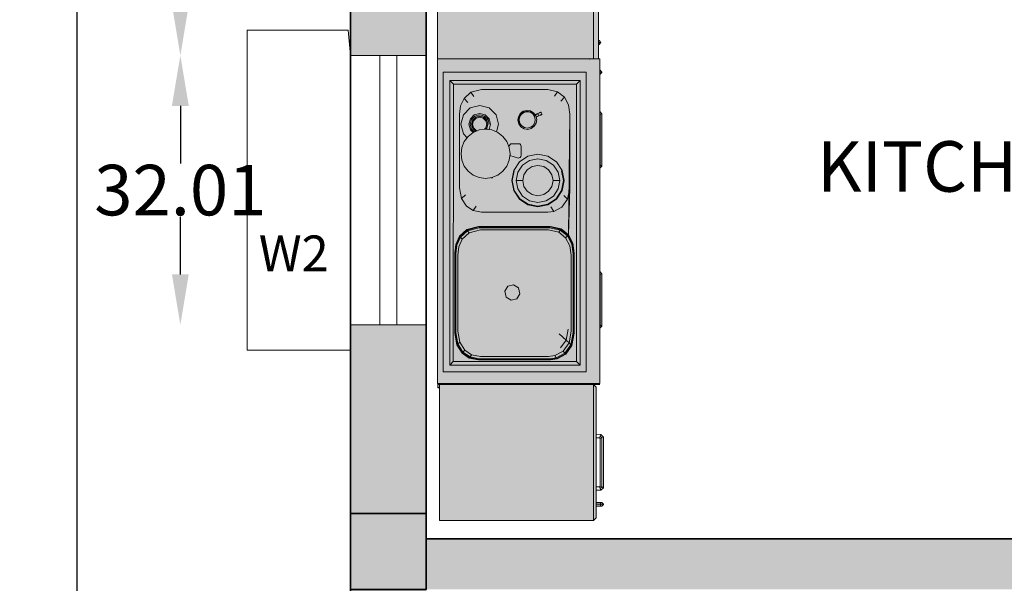
# Model space of a CAD drawing. Units: inches. Extents: x 1994 to 3075, y 3517 to 3950.
# Tile 49 of 58: x 2630 to 2747, y 3656 to 3723. Entities that reach past the tile are written whole.
import ezdxf

# ---------------------------------------------------------------- set-up
doc = ezdxf.new("R2010")
doc.units = ezdxf.units.IN
for name, color, linetype, lineweight in [('A-ANNO-DIMS', 2, 'Continuous', 18), ('A-ANNO-TEXT', 7, 'Continuous', 18), ('A-COLS', 7, 'Continuous', 35), ('A-COLS-PATT', 6, 'Continuous', 13), ('A-FLOR-FIXT', 8, 'Continuous', 18), ('A-GLAZ', 4, 'Continuous', 18), ('A-GLAZ-PROJ', 4, 'Continuous', 18), ('A-WALL', 7, 'Continuous', 35), ('A-WALL-PATT', 252, 'Continuous', 13)]:
    doc.layers.add(name, color=color, linetype=linetype, lineweight=lineweight)
doc.layers.add('hatch', color=254, linetype='Continuous')
doc.styles.get("Standard").update_dxf_attribs({"font": 'arial.ttf'})
doc.dimstyles.get("Standard").update_dxf_attribs({"dimtxt": 6, "dimasz": 6, "dimexe": 0.18, "dimexo": 0.0625, "dimgap": 0.09, "dimtad": 0, "dimtih": 1, "dimtoh": 1, "dimdec": 4, "dimzin": 0, "dimdsep": 46, "dimlunit": 4, "dimtxsty": 'Standard', "dimcen": 0.09, "dimse1": 1, "dimse2": 1, "dimadec": 0, "dimazin": 0, "dimtfac": 1, "dimtdec": 4, "dimtofl": 0, "dimtmove": 0, "dimatfit": 3, "dimfxl": 1, "dimtolj": 1, "dimtzin": 0, "dimarcsym": 0})

# ---------------------------------------------------------------- blocks, each defined once
blk = doc.blocks.new('kithen1')
at = {"layer": 'hatch'}
blk.add_hatch(color=256, dxfattribs=at).paths.add_polyline_path([(-2799.7, -8.3), (-2273.3, -8.3), (-2273.3, -1.7), (-2257.5, -1.7), (-2257.5, -1.1), (-1023.7, -1.1), (-1023.7, 0), (0, 0), (0, -0.3), (0.3, -0.3), (0.3, -1009.9), (-6.1, -1009.9), (-6.1, -2189.3), (-615.8, -2189.3), (-626.5, -2178.9), (-626.5, -1578.2), (-615.8, -1567.8), (-649.5, -1567.8), (-649.5, -1399.1), (-650.3, -1399.1), (-650.3, -1376.8), (-657.9, -1368.5), (-657.8, -1162.4), (-650.3, -1155.1), (-650.3, -1126.4), (-649.5, -1126.4), (-649.5, -1081.1), (-650.3, -1081.1), (-650.3, -1021.1), (-649.5, -1021.1), (-649.5, -959.1), (-651, -959.1), (-650.7, -903), (-653.5, -903), (-660.6, -895.5), (-660.5, -894.6), (-653.5, -887.1), (-651, -887.1), (-651, -638.7), (-651.2, -638.5), (-898.3, -638.5), (-898.3, -640.4), (-905.9, -647.4), (-906.8, -647.4), (-914.3, -640.4), (-914.3, -638.5), (-971.4, -638.5), (-971.4, -642.6), (-1016.2, -642.6), (-1016.2, -643.9), (-1023.8, -650.9), (-1024.7, -650.9), (-1032.2, -643.9), (-1032.2, -642.6), (-1179.7, -642.6), (-1188.8, -650.9), (-1395.6, -650.9), (-1403.7, -642.6), (-1813.5, -642.6), (-1822.6, -650.9), (-2029.4, -650.9), (-2037.5, -642.6), (-2257.5, -642.6), (-2257.5, -618.1), (-2261.3, -618.1), (-2271.7, -628.7), (-2458, -628.7), (-2727.7, -628.7), (-2727.7, -651.1), (-2735, -658.1), (-2735.9, -658), (-2743.2, -651.1), (-2743.2, -628.7), (-2789.4, -628.7), (-2799.7, -618.1)])
at = {"color": 0}
for p, q in [((0, 0), (-1023.7, 0)), ((-2261.3, -8.3), (-2799.7, -8.3)), ((-2799.7, -8.3), (-2799.7, -618.1)), ((-2273.3, -1.9), (-2273.9, -1.9)), ((-2273.9, -1.9), (-2273.9, -8.3)), ((-2261.3, -1.7), (-2273.3, -1.7)), ((-2273.3, -1.7), (-2273.3, -8.3)), ((-2261.3, -601.6), (-2261.3, -1.7)), ((-2261.3, -618.1), (-2261.3, -8.3)), ((-2261, -8.5), (-2261.3, -8.5)), ((-971.4, -1.1), (-2257.5, -1.1)), ((-2257.5, -1.1), (-2257.5, -642.6)), ((-1023.7, -22.5), (-2210.1, -22.5)), ((-2210.1, -22.5), (-2210.1, -589.1)), ((-1023.7, -589.1), (-1023.7, -22.5)), ((-971.4, -1.1), (-971.4, -600.9)), ((-2257.5, -51.5), (-2261.3, -51.5)), ((-2261.3, -51.5), (-2261.3, -536.3)), ((-2183.7, -48.8), (-1056.9, -48.9)), ((-2169.4, -62.7), (-2183.7, -48.8)), ((-2183.7, -48.8), (-2183.7, -565)), ((-2169.7, -550.2), (-2169.4, -62.7)), ((-1071, -63.6), (-2169.4, -62.7)), ((-2103.6, -76.6), (-2136.6, -97.6)), ((-2057.7, -68.5), (-2103.6, -76.6)), ((-2102.3, -78.1), (-2056.8, -70)), ((-2055, -72.6), (-2100.1, -80.6)), ((-1740.9, -68.5), (-2057.7, -68.5)), ((-2056.8, -70), (-1741.9, -70)), ((-1743.7, -72.6), (-2055, -72.6)), ((-1709.7, -76.9), (-1743.7, -72.6)), ((-1741.9, -70), (-1707.6, -74.4)), ((-1706.4, -72.9), (-1740.9, -68.5)), ((-1678, -91.5), (-1709.7, -76.9)), ((-1707.6, -74.4), (-1675.5, -89.1)), ((-1674.1, -87.7), (-1706.4, -72.9)), ((-1056.9, -48.9), (-1071, -63.6)), ((-1071, -550.2), (-1071, -63.6)), ((-1056.9, -48.9), (-1056.9, -565)), ((-2136.6, -97.6), (-2156.1, -126.2)), ((-2154.5, -127.3), (-2135.1, -98.9)), ((-2132.5, -101.2), (-2151.7, -129.3)), ((-2124.5, -108.2), (-2143, -135.3)), ((-2135.1, -98.9), (-2102.3, -78.1)), ((-2132.5, -101.2), (-2135.1, -98.9)), ((-2100.1, -80.6), (-2132.5, -101.2)), ((-2124.5, -108.2), (-2132.5, -101.2)), ((-2093.2, -88.3), (-2124.5, -108.2)), ((-2100.1, -80.6), (-2102.3, -78.1)), ((-2093.2, -88.3), (-2100.1, -80.6)), ((-2049.7, -80.6), (-2093.2, -88.3)), ((-1749, -80.6), (-2049.7, -80.6)), ((-1716.2, -84.8), (-1749, -80.6)), ((-1685.6, -98.8), (-1716.2, -84.8)), ((-1678, -91.5), (-1685.6, -98.8)), ((-1685.6, -98.8), (-1660.4, -125.8)), ((-1651.9, -119.5), (-1678, -91.5)), ((-1675.5, -89.1), (-1649.1, -117.4)), ((-1647.6, -116.2), (-1674.1, -87.7)), ((-1635.3, -163.2), (-1647.6, -116.2)), ((-1554, -114.9), (-1572, -141.2)), ((-1523.7, -95.6), (-1554, -114.9)), ((-1481.5, -88.1), (-1523.7, -95.6)), ((-1523.7, -95.6), (-1509.8, -111.1)), ((-1189.8, -88.1), (-1481.5, -88.1)), ((-1416.2, -122.1), (-1396, -106.6)), ((-1396, -106.6), (-1372.5, -96.9)), ((-1372.5, -96.9), (-1347.3, -93.6)), ((-1347.3, -93.6), (-1322, -96.9)), ((-1322, -96.9), (-1298.5, -106.6)), ((-1298.5, -106.6), (-1278.3, -122.1)), ((-1283.4, -118.2), (-1268.1, -102.9)), ((-1268.1, -102.9), (-1230.5, -92.9)), ((-1230.5, -92.9), (-1193, -102.9)), ((-1193, -102.9), (-1165.5, -130.3)), ((-1157.9, -92.2), (-1189.8, -88.1)), ((-1128.2, -105.8), (-1157.9, -92.2)), ((-1143.5, -120.5), (-1128.2, -105.8)), ((-1128.2, -105.8), (-1103.8, -132)), ((-2156.1, -126.2), (-2163.3, -163.2)), ((-2161.7, -164.1), (-2154.5, -127.3)), ((-2151.7, -129.3), (-2158.8, -165.7)), ((-2151.7, -129.3), (-2154.5, -127.3)), ((-2143, -135.3), (-2151.7, -129.3)), ((-2149.9, -170.5), (-2143, -135.3)), ((-1660.4, -125.8), (-1651.9, -119.5)), ((-1648.8, -170.4), (-1660.4, -125.8)), ((-1649.1, -117.4), (-1651.9, -119.5)), ((-1651.9, -119.5), (-1639.9, -165.7)), ((-1649.1, -117.4), (-1637, -164.1)), ((-1572, -141.2), (-1578.6, -175.3)), ((-1572, -141.2), (-1554.6, -153.3)), ((-1441.5, -165.7), (-1431.7, -142.2)), ((-1431.7, -142.2), (-1416.2, -122.1)), ((-1278.3, -122.1), (-1262.8, -142.2)), ((-1252, -130.7), (-1263.1, -141.8)), ((-1262.8, -142.2), (-1253, -165.7)), ((-1249.5, -134.9), (-1261, -146.4)), ((-1258.4, -151.7), (-1258.6, -152.3)), ((-1246.6, -139.9), (-1258.4, -151.7)), ((-1255.2, -153.5), (-1258.4, -151.7)), ((-1255.2, -153.5), (-1256.4, -157.6)), ((-1244.8, -143), (-1255.2, -153.5)), ((-1252, -130.7), (-1230.5, -124.9)), ((-1249.5, -134.9), (-1230.5, -129.8)), ((-1230.5, -135.6), (-1246.6, -139.9)), ((-1246.6, -139.9), (-1244.8, -143)), ((-1244.8, -143), (-1230.5, -139.2)), ((-1230.5, -124.9), (-1209.1, -130.7)), ((-1230.5, -129.8), (-1211.6, -134.9)), ((-1214.5, -139.9), (-1230.5, -135.6)), ((-1230.5, -135.6), (-1230.5, -139.2)), ((-1230.5, -139.2), (-1216.3, -143)), ((-1216.3, -143), (-1214.5, -139.9)), ((-1205.8, -153.5), (-1216.3, -143)), ((-1211.6, -134.9), (-1214.5, -139.9)), ((-1214.5, -139.9), (-1202.7, -151.7)), ((-1211.6, -134.9), (-1197.7, -148.8)), ((-1209.1, -130.7), (-1193.4, -146.3)), ((-1202.7, -151.7), (-1205.8, -153.5)), ((-1205.8, -153.5), (-1202, -167.7)), ((-1198.4, -167.7), (-1202.7, -151.7)), ((-1197.7, -148.8), (-1192.6, -167.7)), ((-1193.4, -146.3), (-1187.6, -167.7)), ((-1165.5, -130.3), (-1155.5, -167.7)), ((-1103.8, -132), (-1120.8, -144.8)), ((-1103.8, -132), (-1092.5, -175.3)), ((-2163.3, -163.2), (-2163.3, -447.5)), ((-2161.7, -446.6), (-2161.7, -164.1)), ((-2158.8, -165.7), (-2158.8, -445)), ((-2149.9, -440.2), (-2149.9, -170.5)), ((-1648.8, -440.2), (-1648.8, -170.4)), ((-1639.9, -165.7), (-1639.9, -445)), ((-1637, -164.1), (-1637, -446.6)), ((-1635.3, -447.4), (-1635.3, -163.2)), ((-1578.6, -175.3), (-1578.6, -437)), ((-1444.8, -190.8), (-1441.5, -165.7)), ((-1441.5, -216), (-1444.8, -190.8)), ((-1253, -165.7), (-1249.7, -190.8)), ((-1249.7, -190.8), (-1253, -216)), ((-1250.2, -186.9), (-1244.8, -192.3)), ((-1246.6, -195.5), (-1249.9, -192.2)), ((-1244.8, -192.3), (-1246.6, -195.5)), ((-1230.5, -196.1), (-1244.8, -192.3)), ((-1216.3, -192.3), (-1230.5, -196.1)), ((-1205.8, -181.9), (-1216.3, -192.3)), ((-1216.3, -192.3), (-1214.5, -195.5)), ((-1214.5, -195.5), (-1202.7, -183.7)), ((-1197.7, -186.6), (-1211.6, -200.5)), ((-1193.4, -189.1), (-1209.1, -204.7)), ((-1202, -167.7), (-1205.8, -181.9)), ((-1205.8, -181.9), (-1202.7, -183.7)), ((-1202.7, -183.7), (-1198.4, -167.7)), ((-1202, -167.7), (-1198.4, -167.7)), ((-1192.6, -167.7), (-1197.7, -186.6)), ((-1187.6, -167.7), (-1193.4, -189.1)), ((-1155.5, -167.7), (-1165.5, -205.1)), ((-1092.5, -175.3), (-1092.5, -437)), ((-1442, -212), (-1442.1, -213.6)), ((-1442.1, -213.6), (-1441.9, -216.3)), ((-1441.9, -216.3), (-1441.5, -218.2)), ((-1431.7, -239.4), (-1441.5, -216)), ((-1441.5, -218.2), (-1440.8, -218.9)), ((-1440.8, -218.9), (-1440.3, -218.9)), ((-1253, -216), (-1262.8, -239.4)), ((-1230.5, -210.4), (-1251.6, -204.8)), ((-1250.8, -199.1), (-1249.5, -200.5)), ((-1230.5, -199.7), (-1246.6, -195.5)), ((-1214.5, -195.5), (-1230.5, -199.7)), ((-1230.5, -196.1), (-1230.5, -199.7)), ((-1211.6, -200.5), (-1230.5, -205.5)), ((-1209.1, -204.7), (-1230.5, -210.4)), ((-1193, -232.5), (-1230.5, -242.5)), ((-1211.6, -200.5), (-1214.5, -195.5)), ((-1165.5, -205.1), (-1193, -232.5)), ((-1914.6, -272.1), (-1926.9, -292)), ((-1891.8, -266.6), (-1914.6, -272.1)), ((-1871.8, -278.8), (-1891.8, -266.6)), ((-1416.2, -259.6), (-1431.7, -239.4)), ((-1396, -275), (-1416.2, -259.6)), ((-1278.3, -259.6), (-1298.5, -275)), ((-1262.8, -239.4), (-1278.3, -259.6)), ((-1230.5, -242.5), (-1260.7, -234.4)), ((-1926.9, -292), (-1921.4, -314.8)), ((-1878.5, -321.5), (-1866.3, -301.6)), ((-1866.3, -301.6), (-1871.8, -278.8)), ((-1526.8, -324.6), (-1493.1, -302.1)), ((-1493.1, -302.2), (-1526.8, -324.6)), ((-1492.2, -304.2), (-1525.2, -326.2)), ((-1493.1, -302.1), (-1453.2, -294.2)), ((-1453.2, -294.3), (-1493.1, -302.2)), ((-1453.2, -296.5), (-1492.2, -304.2)), ((-1453.2, -311.7), (-1486.4, -318.2)), ((-1453.2, -294.2), (-1413.4, -302.1)), ((-1413.4, -302.2), (-1453.2, -294.3)), ((-1453.2, -294.3), (-1453.2, -296.5)), ((-1453.2, -296.5), (-1414.2, -304.2)), ((-1453.2, -311.7), (-1420.1, -318.2)), ((-1453.2, -338.2), (-1453.2, -311.7)), ((-1413.4, -302.1), (-1379.6, -324.6)), ((-1379.6, -324.6), (-1413.4, -302.2)), ((-1372.5, -284.8), (-1396, -275)), ((-1347.3, -288.1), (-1372.5, -284.8)), ((-1364, -321.4), (-1354.5, -287.1)), ((-1322, -284.8), (-1347.3, -288.1)), ((-1298.5, -275), (-1322, -284.8)), ((-1316.5, -282.5), (-1307.2, -290.8)), ((-1307.2, -290.8), (-1307.2, -321.4)), ((-1921.4, -314.8), (-1901.4, -327)), ((-1901.4, -327), (-1878.5, -321.5)), ((-1526.8, -324.6), (-1549.4, -358.3)), ((-1549.4, -358.3), (-1526.8, -324.6)), ((-1525.2, -326.2), (-1547.3, -359.2)), ((-1514.5, -337), (-1533.3, -365)), ((-1486.4, -318.2), (-1514.5, -337)), ((-1495.7, -355.7), (-1476.2, -342.8)), ((-1476.2, -342.8), (-1453.2, -338.2)), ((-1430.3, -342.8), (-1453.2, -338.2)), ((-1410.8, -355.7), (-1430.3, -342.8)), ((-1420.1, -318.2), (-1392, -337)), ((-1392, -337), (-1373.2, -365)), ((-1379.6, -324.6), (-1357, -358.3)), ((-1357, -358.3), (-1379.6, -324.6)), ((-1363.6, -324.3), (-1364, -321.4)), ((-1361.6, -328), (-1363.6, -324.3)), ((-1357.9, -330.6), (-1361.6, -328)), ((-1352.7, -331.6), (-1357.9, -330.6)), ((-1318.5, -331.6), (-1352.7, -331.6)), ((-1314.3, -331), (-1318.5, -331.6)), ((-1310.7, -329.1), (-1314.3, -331)), ((-1308.2, -326), (-1310.7, -329.1)), ((-1307.2, -321.4), (-1308.2, -326)), ((-1250.4, -357.6), (-1248.3, -343.1)), ((-1248.3, -343.1), (-1240.7, -330.6)), ((-1245.1, -357.3), (-1243.2, -344.9)), ((-1243.2, -344.9), (-1236.8, -334.2)), ((-1240.7, -330.6), (-1228.9, -321.9)), ((-1227.6, -324.8), (-1238.3, -332.8)), ((-1236.8, -334.2), (-1226.7, -326.8)), ((-1228.9, -321.9), (-1214.7, -318.4)), ((-1227.6, -324.8), (-1228.3, -323.3)), ((-1214.6, -321.6), (-1227.6, -324.8)), ((-1226.7, -326.8), (-1214.5, -323.7)), ((-1214.7, -318.4), (-1200.3, -320.6)), ((-1214.7, -319.9), (-1214.6, -321.6)), ((-1214.6, -321.6), (-1201.4, -323.6)), ((-1214.5, -323.7), (-1202.1, -325.6)), ((-1202.1, -325.6), (-1191.3, -332)), ((-1201.4, -323.6), (-1200.8, -322)), ((-1201.4, -323.6), (-1189.9, -330.5)), ((-1200.3, -320.6), (-1187.7, -328.1)), ((-1191.3, -332), (-1183.9, -342.1)), ((-1189.9, -330.5), (-1188.7, -329.2)), ((-1189.9, -330.5), (-1181.9, -341.2)), ((-1187.7, -328.1), (-1179, -339.8)), ((-1183.9, -342.1), (-1180.8, -354.2)), ((-1181.9, -341.2), (-1180.4, -340.5)), ((-1181.9, -341.2), (-1178.7, -354.1)), ((-1179, -339.8), (-1175.5, -354)), ((-1549.4, -358.3), (-1557.3, -398)), ((-1557.3, -398), (-1549.4, -358.3)), ((-1547.3, -359.2), (-1555.1, -398)), ((-1533.3, -365), (-1539.9, -398)), ((-1513.2, -398), (-1508.7, -375.1)), ((-1508.7, -375.1), (-1495.7, -355.7)), ((-1397.8, -375.1), (-1410.8, -355.7)), ((-1393.2, -398), (-1397.8, -375.1)), ((-1373.2, -365), (-1366.6, -398)), ((-1357, -358.3), (-1349.1, -398)), ((-1349.1, -398), (-1357, -358.3)), ((-1246.9, -371.7), (-1250.4, -357.6)), ((-1238.2, -383.5), (-1246.9, -371.7)), ((-1242, -369.4), (-1245.1, -357.3)), ((-1234.6, -379.5), (-1242, -369.4)), ((-1225.6, -391), (-1238.2, -383.5)), ((-1223.8, -385.9), (-1234.6, -379.5)), ((-1211.4, -387.8), (-1223.8, -385.9)), ((-1199.2, -384.8), (-1211.4, -387.8)), ((-1197, -389.6), (-1211.2, -393.1)), ((-1189.2, -377.3), (-1199.2, -384.8)), ((-1187.6, -378.8), (-1198.3, -386.7)), ((-1185.2, -380.9), (-1197, -389.6)), ((-1193.3, -386.9), (-1194.2, -387.6)), ((-1193.1, -386.7), (-1193.3, -386.9)), ((-1193.3, -386.9), (-1191.3, -391.2)), ((-1192.7, -386.5), (-1192.9, -386.6)), ((-1192.6, -386.8), (-1192.7, -386.5)), ((-1190.5, -391.2), (-1192.6, -386.8)), ((-1182.7, -366.6), (-1189.2, -377.3)), ((-1180.7, -367.3), (-1187.6, -378.8)), ((-1187.6, -378.8), (-1186.3, -379.9)), ((-1177.6, -368.4), (-1185.2, -380.9)), ((-1180.8, -354.2), (-1182.7, -366.6)), ((-1178.7, -354.1), (-1180.7, -367.3)), ((-1180.7, -367.3), (-1179.1, -367.9)), ((-1178.7, -354.1), (-1177, -354.1)), ((-1175.5, -354), (-1177.6, -368.4)), ((-1557.3, -398), (-1549.4, -437.8)), ((-1549.4, -437.8), (-1557.3, -398)), ((-1555.1, -398), (-1547.3, -436.9)), ((-1539.9, -398), (-1533.3, -431.1)), ((-1508.7, -420.9), (-1513.2, -398)), ((-1495.7, -440.4), (-1508.7, -420.9)), ((-1410.8, -440.4), (-1397.8, -420.9)), ((-1397.8, -420.9), (-1393.2, -398)), ((-1366.6, -398), (-1373.2, -431.1)), ((-1349.1, -398), (-1357, -437.8)), ((-1357, -437.8), (-1349.1, -398)), ((-1211.2, -393.1), (-1225.6, -391)), ((-1202.1, -390.9), (-1202.4, -391)), ((-1202.4, -391), (-1202, -390.9)), ((-1202.4, -391), (-1202.4, -391)), ((-1202.4, -391), (-1202.3, -391.3)), ((-1202.3, -391.3), (-1200.2, -395.7)), ((-1202, -390.9), (-1202.1, -390.9)), ((-1201.7, -390.8), (-1199.7, -395.1)), ((-1200.2, -395.7), (-1199.7, -395.1)), ((-1200.2, -395.7), (-1197.3, -401.8)), ((-1199.7, -395.1), (-1198, -394.1)), ((-1199.7, -395.1), (-1196.7, -401.5)), ((-1197.3, -401.8), (-1196.7, -401.5)), ((-1197.3, -401.8), (-1194.5, -407.8)), ((-1196.7, -401.5), (-1190.1, -398.4)), ((-1196.7, -401.5), (-1193.7, -407.8)), ((-1194.5, -407.8), (-1193.7, -407.8)), ((-1192.4, -412.2), (-1194.5, -407.8)), ((-1193.7, -407.8), (-1191.8, -407.2)), ((-1193.7, -407.8), (-1191.5, -412.5)), ((-1191.3, -391.2), (-1193.2, -391.8)), ((-1191.6, -413.9), (-1192.4, -412.2)), ((-1190.7, -414.2), (-1191.6, -413.9)), ((-1191.3, -391.2), (-1190.5, -391.2)), ((-1188.3, -397.5), (-1191.3, -391.2)), ((-1188.7, -413.8), (-1190.7, -414.2)), ((-1190.5, -391.2), (-1187.6, -397.2)), ((-1190.1, -398.4), (-1188.3, -397.5)), ((-1186.2, -412.8), (-1188.7, -413.8)), ((-1187.6, -397.2), (-1188.3, -397.5)), ((-1188.3, -397.5), (-1185.3, -403.9)), ((-1184.8, -403.3), (-1187.6, -397.2)), ((-1185.3, -403.9), (-1186.9, -404.9)), ((-1183.8, -411.5), (-1186.2, -412.8)), ((-1185.3, -403.9), (-1184.8, -403.3)), ((-1183.1, -408.5), (-1185.3, -403.9)), ((-1184.8, -403.3), (-1182.7, -407.7)), ((-1182.3, -410.2), (-1183.8, -411.5)), ((-1182.7, -407.7), (-1181.9, -409.3)), ((-1181.9, -409.3), (-1182.3, -410.2)), ((-2163.3, -447.5), (-2159.9, -473.6)), ((-2158.2, -472.6), (-2161.7, -446.6)), ((-2158.8, -445), (-2155.4, -470.7)), ((-2155.4, -470.7), (-2146.6, -465)), ((-2146.6, -465), (-2149.9, -440.2)), ((-2146.6, -465), (-2128.8, -498)), ((-1658, -480.4), (-1648.8, -440.2)), ((-1639.9, -445), (-1649.4, -486.6)), ((-1637, -446.6), (-1646.6, -488.6)), ((-1645, -489.8), (-1635.3, -447.4)), ((-1578.6, -437), (-1575.5, -461.1)), ((-1575.5, -461.1), (-1557.8, -449.7)), ((-1575.5, -461.1), (-1558.2, -493)), ((-1549.4, -437.8), (-1526.8, -471.4)), ((-1526.8, -471.4), (-1549.4, -437.8)), ((-1547.3, -436.9), (-1525.2, -469.8)), ((-1533.3, -431.1), (-1514.5, -459.1)), ((-1514.5, -459.1), (-1486.4, -477.9)), ((-1476.2, -453.3), (-1495.7, -440.4)), ((-1453.2, -457.9), (-1476.2, -453.3)), ((-1453.2, -457.9), (-1430.3, -453.3)), ((-1453.2, -484.4), (-1453.2, -457.9)), ((-1430.3, -453.3), (-1410.8, -440.4)), ((-1392, -459.1), (-1420.1, -477.9)), ((-1373.2, -431.1), (-1392, -459.1)), ((-1357, -437.8), (-1379.6, -471.4)), ((-1379.6, -471.4), (-1357, -437.8)), ((-1101.4, -476), (-1118.7, -463.5)), ((-1092.5, -437), (-1101.4, -476)), ((-2159.9, -473.6), (-2141.1, -508.3)), ((-2139.6, -507.1), (-2158.2, -472.6)), ((-2137, -504.8), (-2155.4, -470.7)), ((-2137, -504.8), (-2139.6, -507.1)), ((-2128.8, -498), (-2137, -504.8)), ((-2103.3, -528.8), (-2137, -504.8)), ((-2128.8, -498), (-2096.3, -521.1)), ((-2085.5, -509.3), (-2116.3, -487.4)), ((-2060.9, -482.3), (-2085.5, -509.3)), ((-1680.2, -507.9), (-1658, -480.4)), ((-1649.4, -486.6), (-1672.5, -515.1)), ((-1646.6, -488.6), (-1669.9, -517.4)), ((-1668.5, -518.8), (-1645, -489.8)), ((-1649.4, -486.6), (-1658, -480.4)), ((-1646.6, -488.6), (-1649.4, -486.6)), ((-1558.2, -493), (-1526.7, -515.5)), ((-1493.1, -493.9), (-1526.8, -471.4)), ((-1526.8, -471.4), (-1493.1, -493.9)), ((-1526.7, -515.5), (-1512.6, -500.1)), ((-1525.2, -469.8), (-1492.2, -491.9)), ((-1453.2, -501.8), (-1493.1, -493.9)), ((-1493.1, -493.9), (-1453.2, -501.8)), ((-1492.2, -491.9), (-1453.2, -499.6)), ((-1486.4, -477.9), (-1453.2, -484.4)), ((-1420.1, -477.9), (-1453.2, -484.4)), ((-1453.2, -499.6), (-1414.2, -491.9)), ((-1413.4, -493.9), (-1453.2, -501.8)), ((-1453.2, -501.8), (-1413.4, -493.9)), ((-1453.2, -499.6), (-1453.2, -501.8)), ((-1379.6, -471.4), (-1413.4, -493.9)), ((-1413.4, -493.9), (-1379.6, -471.4)), ((-1123, -502.7), (-1153.4, -518.8)), ((-1123, -502.7), (-1138.7, -488.2)), ((-1101.4, -476), (-1123, -502.7)), ((-2257.5, -535.3), (-2257.9, -535.3)), ((-2141.1, -508.3), (-2106.9, -532.7)), ((-2105.6, -531.3), (-2139.6, -507.1)), ((-2106.9, -532.7), (-2057.7, -542.2)), ((-2103.3, -528.8), (-2105.6, -531.3)), ((-2056.8, -540.7), (-2105.6, -531.3)), ((-2096.3, -521.1), (-2103.3, -528.8)), ((-2055, -538.1), (-2103.3, -528.8)), ((-2096.3, -521.1), (-2085.5, -509.3)), ((-2049.7, -530.1), (-2096.3, -521.1)), ((-2085.5, -509.3), (-2041.5, -517.8)), ((-2057.7, -542.2), (-2056.8, -540.7)), ((-1783.5, -542.2), (-2057.7, -542.2)), ((-1781.7, -540.7), (-2056.8, -540.7)), ((-1778.6, -538.1), (-2055, -538.1)), ((-1749, -530.1), (-2049.7, -530.1)), ((-1749, -530.1), (-1797.1, -530.1)), ((-1743.7, -538.1), (-1797.1, -538.1)), ((-1741.9, -540.7), (-1797.1, -540.7)), ((-1740.9, -542.2), (-1797.1, -542.2)), ((-1711.5, -524.5), (-1749, -530.1)), ((-1704.9, -532.3), (-1743.7, -538.1)), ((-1741.9, -540.7), (-1702.7, -534.9)), ((-1740.9, -542.2), (-1741.9, -540.7)), ((-1701.5, -536.3), (-1740.9, -542.2)), ((-1680.2, -507.9), (-1711.5, -524.5)), ((-1672.5, -515.1), (-1704.9, -532.3)), ((-1702.7, -534.9), (-1669.9, -517.4)), ((-1668.5, -518.8), (-1701.5, -536.3)), ((-1672.5, -515.1), (-1680.2, -507.9)), ((-1669.9, -517.4), (-1672.5, -515.1)), ((-1189.8, -524.2), (-1668.5, -518.8)), ((-1481.5, -524.2), (-1668.5, -518.8)), ((-1526.7, -515.5), (-1481.5, -524.2)), ((-1189.8, -524.2), (-1481.5, -524.2)), ((-1153.4, -518.8), (-1189.8, -524.2)), ((-2183.7, -565), (-2169.7, -550.2)), ((-1797.1, -565), (-2183.7, -565)), ((-1793.1, -550.2), (-2169.7, -550.2)), ((-1071, -550.2), (-1797.1, -550.2)), ((-1056.9, -565), (-1797.1, -565)), ((-1056.9, -565), (-1071, -550.2)), ((-2799.7, -618.1), (-2261.3, -618.1)), ((-2789.4, -628.7), (-2799.7, -618.1)), ((-2261.3, -618.1), (-2271.7, -628.7)), ((-2261, -596.4), (-2261.3, -596.4)), ((-2261.3, -626.3), (-2261.3, -601.6)), ((-2210.1, -589.1), (-1789.4, -589.1)), ((-1797.1, -589.1), (-1023.7, -589.1)), ((-972.7, -601.6), (-972.7, -603)), ((-971.4, -600.6), (-971.4, -601.6)), ((-971.4, -603), (-971.4, -642.6)), ((-630.9, -618.1), (-971.4, -618.1)), ((-2271.7, -628.7), (-2789.4, -628.7)), ((-2743.2, -628.7), (-2743.2, -644.8)), ((-2743.2, -644.8), (-2742.3, -644.5)), ((-2743.2, -651.1), (-2743.2, -644.8)), ((-2742.3, -650.3), (-2743.2, -651.1)), ((-2742.3, -651.1), (-2743.2, -651.1)), ((-2743.2, -651.1), (-2735.9, -658)), ((-2742.3, -628.7), (-2742.3, -644.4)), ((-2742.3, -644.4), (-2734.9, -647.4)), ((-2742.3, -644.4), (-2742.3, -651.1)), ((-2735, -658.1), (-2742.3, -651.1)), ((-2735.9, -658), (-2735, -658.1)), ((-2734.9, -647.4), (-2735, -658.1)), ((-2735, -658.1), (-2727.7, -651.1)), ((-2734.9, -647.4), (-2734.9, -628.7)), ((-2727.7, -644.4), (-2734.9, -647.4)), ((-2727.7, -628.7), (-2727.7, -644.4)), ((-2727.7, -651.1), (-2727.7, -644.4)), ((-2679.7, -628.7), (-2679.4, -647.7)), ((-2679.4, -647.7), (-2665.9, -642)), ((-2669.5, -658), (-2679.4, -647.7)), ((-2666.7, -651.1), (-2672.6, -644.8)), ((-2666.7, -651.1), (-2669.5, -658)), ((-2669.5, -658), (-2469.7, -658.1)), ((-2663.9, -644.2), (-2666.7, -651.1)), ((-2472.3, -651.1), (-2666.7, -651.1)), ((-2665.6, -628.7), (-2665.9, -642)), ((-2665.9, -642), (-2663.9, -644.2)), ((-2663.9, -644.2), (-2474.9, -644.1)), ((-2474.9, -644.1), (-2471.7, -641.3)), ((-2474.9, -644.1), (-2472.3, -651.1)), ((-2472.3, -651.1), (-2465, -644.4)), ((-2469.7, -658.1), (-2472.3, -651.1)), ((-2471.7, -641.3), (-2472, -628.7)), ((-2458.4, -647.4), (-2471.7, -641.3)), ((-2458.4, -647.4), (-2469.7, -658.1)), ((-2458, -628.7), (-2458.4, -647.4)), ((-2261.3, -643.6), (-2261.3, -626.3)), ((-2257.5, -642.6), (-1797.1, -642.6)), ((-2037.5, -642.6), (-2029.4, -650.9)), ((-2029.4, -650.9), (-2026.5, -643.9)), ((-2029.4, -650.9), (-1828.9, -650.9)), ((-2026.5, -643.9), (-2027.8, -642.6)), ((-2025.9, -642.6), (-2026.5, -643.9)), ((-2026.5, -643.9), (-1828.9, -643.9)), ((-1825.3, -643.9), (-1828.9, -643.9)), ((-1822.6, -650.9), (-1828.9, -650.9)), ((-1825.8, -642.6), (-1825.3, -643.9)), ((-1825.3, -643.9), (-1823.8, -642.6)), ((-1822.6, -650.9), (-1825.3, -643.9)), ((-1813.5, -642.6), (-1822.6, -650.9)), ((-971.4, -642.6), (-1797.1, -642.6)), ((-1395.6, -650.9), (-1403.7, -642.6)), ((-1392.7, -643.9), (-1395.6, -650.9)), ((-1395.6, -650.9), (-1188.8, -650.9)), ((-1394, -642.6), (-1392.7, -643.9)), ((-1392.7, -643.9), (-1392.1, -642.6)), ((-1191.5, -643.9), (-1392.7, -643.9)), ((-1192, -642.6), (-1191.5, -643.9)), ((-1191.5, -643.9), (-1190, -642.6)), ((-1188.8, -650.9), (-1191.5, -643.9)), ((-1179.7, -642.6), (-1188.8, -650.9)), ((-1032.2, -643.9), (-1032.2, -642.6)), ((-1031.4, -643.1), (-1032.2, -643.9)), ((-1031.4, -643.9), (-1032.2, -643.9)), ((-1032.2, -643.9), (-1024.7, -650.9)), ((-1031.4, -642.6), (-1031.4, -643.9)), ((-1023.8, -650.9), (-1031.4, -643.9)), ((-1024.7, -650.9), (-1023.8, -650.9)), ((-1023.8, -650.9), (-1023.8, -642.6)), ((-1016.2, -643.9), (-1023.8, -650.9)), ((-1016.2, -642.6), (-1016.2, -643.9)), ((-971.4, -635.7), (-971.4, -641.8)), ((-971.4, -641.8), (-971.4, -638.3)), ((-651.2, -638.5), (-971.4, -638.5)), ((-914.3, -640.4), (-914.4, -638.5)), ((-913.5, -639.6), (-914.3, -640.4)), ((-913.5, -640.4), (-914.3, -640.4)), ((-914.3, -640.4), (-906.8, -647.3)), ((-913.5, -638.5), (-913.5, -640.4)), ((-905.9, -647.4), (-913.5, -640.4)), ((-906.8, -647.3), (-905.9, -647.4)), ((-905.9, -647.4), (-905.9, -638.5)), ((-898.3, -640.4), (-905.9, -647.4)), ((-898.3, -638.5), (-898.3, -640.4))]:
    blk.add_line(p, q, dxfattribs=at)
for points in [[(-2799.7, -8.3), (-2273.3, -8.3), (-2273.3, -1.7), (-2257.5, -1.7), (-2257.5, -1.1), (-1023.7, -1.1), (-1023.7, 0), (0, 0)], [(-651.2, -638.5), (-898.3, -638.5), (-898.3, -640.4), (-905.9, -647.4), (-906.8, -647.4), (-914.3, -640.4), (-914.3, -638.5), (-971.4, -638.5), (-971.4, -642.6), (-1016.2, -642.6), (-1016.2, -643.9), (-1023.8, -650.9), (-1024.7, -650.9), (-1032.2, -643.9), (-1032.2, -642.6), (-1179.7, -642.6), (-1188.8, -650.9), (-1395.6, -650.9), (-1403.7, -642.6), (-1813.5, -642.6), (-1822.6, -650.9), (-2029.4, -650.9), (-2037.5, -642.6), (-2257.5, -642.6), (-2257.5, -618.1), (-2261.3, -618.1), (-2271.7, -628.7), (-2458, -628.7), (-2727.7, -628.7), (-2727.7, -651.1), (-2735, -658.1), (-2735.9, -658), (-2743.2, -651.1), (-2743.2, -628.7), (-2789.4, -628.7), (-2799.7, -618.1), (-2799.7, -8.3)]]:
    blk.add_lwpolyline(points)
blk = doc.blocks.new('*D29')
at = {"layer": 'A-ANNO-DIMS', "color": 0, "lineweight": -2, "transparency": 16777216}
for p, q in [((2757.66, 3741.43), (2757.66, 3708.56)), ((2757.66, 3669.3), (2757.66, 3702.17))]:
    blk.add_line(p, q, dxfattribs=at)
at = {"layer": 'A-ANNO-DIMS', "color": 0, "transparency": 16777216}
for points in [[(2756.66, 3741.43), (2758.66, 3741.43), (2757.66, 3747.43)], [(2756.66, 3669.3), (2758.66, 3669.3), (2757.66, 3663.3)]]:
    blk.add_solid(points, dxfattribs=at)
at = {"layer": 'Defpoints', "color": 0, "transparency": 16777216}
for p in [(2745.04, 3747.43), (2757.66, 3747.43), (2745.04, 3663.3)]:
    blk.add_point(p, dxfattribs=at)
at = {"layer": 'A-ANNO-DIMS', "color": 0, "transparency": 16777216, "insert": (2757.66, 3705.36), "char_height": 6, "attachment_point": 5}
blk.add_mtext('\\A1;KITCHEN UNIT 84', dxfattribs=at)
blk = doc.blocks.new('*D32')
at = {"layer": 'A-ANNO-DIMS', "color": 0, "lineweight": -2, "transparency": 16777216}
for p, q in [((2636.61, 3908.13), (2636.61, 3730.78)), ((2636.61, 3547.13), (2636.61, 3724.47))]:
    blk.add_line(p, q, dxfattribs=at)
at = {"layer": 'A-ANNO-DIMS', "color": 0, "transparency": 16777216}
for points in [[(2635.61, 3908.13), (2637.61, 3908.13), (2636.61, 3914.13)], [(2635.61, 3547.13), (2637.61, 3547.13), (2636.61, 3541.13)]]:
    blk.add_solid(points, dxfattribs=at)
at = {"layer": 'Defpoints', "color": 0, "transparency": 16777216}
for p in [(2636.61, 3914.13), (2669.07, 3914.13), (2810.07, 3541.13)]:
    blk.add_point(p, dxfattribs=at)
at = {"layer": 'A-ANNO-DIMS', "color": 0, "transparency": 16777216, "insert": (2636.61, 3727.63), "char_height": 6, "attachment_point": 5}
blk.add_mtext('\\A1;373', dxfattribs=at)
blk = doc.blocks.new('*D45')
at = {"layer": 'A-ANNO-DIMS', "color": 0, "lineweight": -2, "transparency": 16777216}
for p, q in [((2648.87, 3712.55), (2648.87, 3705.7)), ((2648.87, 3692.54), (2648.87, 3699.39))]:
    blk.add_line(p, q, dxfattribs=at)
at = {"layer": 'A-ANNO-DIMS', "color": 0, "transparency": 16777216}
for points in [[(2647.87, 3712.55), (2649.87, 3712.55), (2648.87, 3718.55)], [(2647.87, 3692.54), (2649.87, 3692.54), (2648.87, 3686.54)]]:
    blk.add_solid(points, dxfattribs=at)
at = {"layer": 'Defpoints', "color": 0, "transparency": 16777216}
for p in [(2648.87, 3718.55), (2669.07, 3718.55), (2669.07, 3686.54)]:
    blk.add_point(p, dxfattribs=at)
at = {"layer": 'A-ANNO-DIMS', "color": 0, "transparency": 16777216, "insert": (2648.87, 3702.55), "char_height": 6, "attachment_point": 5}
blk.add_mtext('\\A1;32.01', dxfattribs=at)
blk = doc.blocks.new('*D46')
at = {"layer": 'A-ANNO-DIMS', "color": 0, "lineweight": -2, "transparency": 16777216}
for p, q in [((2648.87, 3749.13), (2648.87, 3740)), ((2648.87, 3724.55), (2648.87, 3733.68))]:
    blk.add_line(p, q, dxfattribs=at)
at = {"layer": 'A-ANNO-DIMS', "color": 0, "transparency": 16777216}
for points in [[(2647.87, 3749.13), (2649.87, 3749.13), (2648.87, 3755.13)], [(2647.87, 3724.55), (2649.87, 3724.55), (2648.87, 3718.55)]]:
    blk.add_solid(points, dxfattribs=at)
at = {"layer": 'Defpoints', "color": 0, "transparency": 16777216}
for p in [(2648.87, 3755.13), (2669.07, 3755.13), (2669.07, 3718.55)]:
    blk.add_point(p, dxfattribs=at)
at = {"layer": 'A-ANNO-DIMS', "color": 0, "transparency": 16777216, "insert": (2648.87, 3736.84), "char_height": 6, "attachment_point": 5}
blk.add_mtext('\\A1;36.575', dxfattribs=at)

msp = doc.modelspace()

# ---------------------------------------------------------------- hatches: boundary and pattern name
at = {"layer": 'A-COLS-PATT'}
h = msp.add_hatch(color=256, dxfattribs=at)
h.dxf.hatch_style = 1
h.paths.add_polyline_path([(2678.072, 3914.1269), (2669.072, 3914.1269), (2669.072, 3905.1269), (2678.072, 3905.1269)])
h.paths.add_polyline_path([(2816.072, 3914.1269), (2807.072, 3914.1269), (2807.072, 3905.1269), (2816.072, 3905.1269)])
h.paths.add_polyline_path([(2894.9096, 3914.1269), (2885.9096, 3914.1269), (2885.9096, 3905.1269), (2894.9096, 3905.1269)])
h.paths.add_polyline_path([(3033.072, 3914.1269), (3024.072, 3914.1269), (3024.072, 3905.1269), (3033.072, 3905.1269)])
h.paths.add_polyline_path([(3033.072, 3764.1269), (3024.072, 3764.1269), (3024.072, 3755.1269), (3033.072, 3755.1269)])
h.paths.add_polyline_path([(2895.072, 3764.1269), (2886.072, 3764.1269), (2886.072, 3755.1269), (2895.072, 3755.1269)])
h.paths.add_polyline_path([(2816.072, 3764.1269), (2807.072, 3764.1269), (2807.072, 3755.1269), (2816.072, 3755.1269)])
h.paths.add_polyline_path([(2678.072, 3764.1269), (2669.072, 3764.1269), (2669.072, 3755.1269), (2678.072, 3755.1269)])
h.paths.add_polyline_path([(2678.072, 3664.1269), (2669.072, 3664.1269), (2669.072, 3655.1269), (2678.072, 3655.1269)])
h.paths.add_polyline_path([(2816.072, 3664.1269), (2807.072, 3664.1269), (2807.072, 3655.1269), (2816.072, 3655.1269)])
h.paths.add_polyline_path([(3033.072, 3616.1269), (3024.072, 3616.1269), (3024.072, 3607.1269), (3033.072, 3607.1269)])
h.paths.add_polyline_path([(2894.9096, 3616.1269), (2885.9096, 3616.1269), (2885.9096, 3607.1269), (2894.9096, 3607.1269)])
h.paths.add_polyline_path([(2816.072, 3559.1269), (2807.072, 3559.1269), (2807.072, 3550.1269), (2816.072, 3550.1269)])
h.paths.add_polyline_path([(2678.072, 3559.1269), (2669.072, 3559.1269), (2669.072, 3550.1269), (2678.072, 3550.1269)])
at = {"layer": 'A-WALL-PATT'}
h = msp.add_hatch(color=256, dxfattribs=at)
h.dxf.hatch_style = 1
h.paths.add_polyline_path([(2678.072, 3755.1269), (2669.072, 3755.1269), (2669.072, 3718.5523), (2678.072, 3718.5523)])
h.paths.add_polyline_path([(2807.072, 3761.1269), (2678.072, 3761.1269), (2678.072, 3755.1269), (2807.072, 3755.1269)])
h.paths.add_polyline_path([(2678.072, 3812.7371), (2669.072, 3812.7371), (2669.072, 3809.7371), (2669.072, 3764.1269), (2678.072, 3764.1269)])
h.paths.add_polyline_path([(2678.072, 3905.1269), (2669.072, 3905.1269), (2669.072, 3868.7491), (2678.072, 3868.7491)])
h.paths.add_polyline_path([(2723.826, 3914.1269), (2720.826, 3914.1269), (2678.072, 3914.1269), (2678.072, 3905.1269), (2723.826, 3905.1269)])
h.paths.add_polyline_path([(2807.072, 3914.1269), (2779.838, 3914.1269), (2779.838, 3905.1269), (2807.072, 3905.1269)])
h.paths.add_polyline_path([(2837.6979, 3914.1269), (2834.6979, 3914.1269), (2820.9062, 3914.1269), (2816.072, 3914.1269), (2816.072, 3905.1269), (2837.6979, 3905.1269)])
h.paths.add_polyline_path([(2885.9096, 3914.1269), (2869.71, 3914.1269), (2869.71, 3905.1269), (2876.9183, 3905.1269), (2885.9096, 3905.1269)])
h.paths.add_polyline_path([(2933.6904, 3914.1269), (2930.6904, 3914.1269), (2894.9096, 3914.1269), (2894.9096, 3905.1269), (2933.6904, 3905.1269)])
h.paths.add_polyline_path([(3024.072, 3914.1269), (2989.7025, 3914.1269), (2989.7025, 3905.1269), (3024.072, 3905.1269)])
h.paths.add_polyline_path([(3033.072, 3905.1269), (3024.072, 3905.1269), (3024.072, 3861.4192), (3033.072, 3861.4192)])
h.paths.add_polyline_path([(3033.072, 3805.4072), (3024.072, 3805.4072), (3024.072, 3764.1269), (3033.072, 3764.1269)])
h.paths.add_polyline_path([(3033.072, 3755.1269), (3024.072, 3755.1269), (3024.072, 3732.1247), (3033.072, 3732.1247), (3033.072, 3735.1247)])
h.paths.add_polyline_path([(3024.072, 3761.1269), (2895.072, 3761.1269), (2895.072, 3755.1269), (3024.072, 3755.1269)])
h.paths.add_polyline_path([(3033.072, 3676.1126), (3024.072, 3676.1126), (3024.072, 3616.1269), (3033.072, 3616.1269)])
h.paths.add_polyline_path([(3024.072, 3613.1269), (2959.4908, 3613.1269), (2959.4908, 3607.1269), (3024.072, 3607.1269)])
h.paths.add_polyline_path([(2914.1254, 3613.1269), (2894.9096, 3613.1269), (2894.9096, 3607.1269), (2914.1254, 3607.1269)])
h.paths.add_polyline_path([(2885.9096, 3613.1269), (2852.072, 3613.1269), (2852.072, 3607.1269), (2885.9096, 3607.1269)])
h.paths.add_polyline_path([(2822.072, 3613.1269), (2810.072, 3613.1269), (2810.072, 3559.1269), (2816.072, 3559.1269), (2816.072, 3607.1269), (2822.072, 3607.1269)])
h.paths.add_polyline_path([(2933.072, 3607.1269), (2924.072, 3607.1269), (2924.072, 3550.1269), (2892.072, 3550.1269), (2816.072, 3550.1269), (2810.072, 3550.1269), (2810.072, 3541.1269), (2892.072, 3541.1269), (2933.072, 3541.1269)])
h.paths.add_polyline_path([(2807.072, 3559.1269), (2678.072, 3559.1269), (2678.072, 3550.1269), (2807.072, 3550.1269)])
h.paths.add_polyline_path([(2678.072, 3655.1269), (2669.072, 3655.1269), (2669.072, 3559.1269), (2678.072, 3559.1269)])
h.paths.add_polyline_path([(2678.072, 3686.5403), (2669.072, 3686.5403), (2669.072, 3664.1269), (2678.072, 3664.1269)])
h.paths.add_polyline_path([(2807.072, 3661.1269), (2678.072, 3661.1269), (2678.072, 3655.1269), (2807.072, 3655.1269)])
h.paths.add_polyline_path([(2816.072, 3755.1269), (2810.072, 3755.1269), (2810.072, 3703.1269), (2816.072, 3703.1269)])
h.paths.add_polyline_path([(2816.072, 3905.1269), (2810.072, 3905.1269), (2810.072, 3803.1269), (2816.072, 3803.1269), (2816.072, 3815.1269)])
h.paths.add_polyline_path([(2886.072, 3821.1269), (2852.072, 3821.1269), (2852.072, 3815.1269), (2886.072, 3815.1269)])
h.paths.add_polyline_path([(2822.072, 3821.1269), (2816.072, 3821.1269), (2816.072, 3815.1269), (2822.072, 3815.1269)])
h.paths.add_polyline_path([(2892.072, 3905.1269), (2886.072, 3905.1269), (2886.072, 3803.1269), (2892.072, 3803.1269)])

# ---------------------------------------------------------------- linework, layer by layer
at = {"layer": 'A-COLS'}
msp.add_lwpolyline([(2669.072, 3655.1269), (2678.072, 3655.1269), (2678.072, 3664.1269), (2669.072, 3664.1269)], close=True, dxfattribs=at)
at = {"layer": 'A-GLAZ'}
for p, q in [((2678.072, 3718.5523), (2669.072, 3718.5523)), ((2672.572, 3718.5523), (2672.572, 3686.5403)), ((2674.572, 3718.5523), (2674.572, 3686.5403)), ((2669.072, 3686.5403), (2678.072, 3686.5403))]:
    msp.add_line(p, q, dxfattribs=at)
at = {"layer": 'A-GLAZ-PROJ'}
for p, q in [((2668.8096, 3721.5408), (2656.8096, 3721.5408)), ((2656.8096, 3721.5408), (2656.8096, 3686.5403)), ((2669.072, 3718.5523), (2668.8096, 3721.5408)), ((2656.8096, 3686.5403), (2656.8096, 3683.5403)), ((2656.8096, 3683.5403), (2669.072, 3683.5403))]:
    msp.add_line(p, q, dxfattribs=at)
at = {"layer": 'A-WALL'}
for p, q in [((2669.072, 3914.1269), (2669.072, 3550.1269)), ((2678.072, 3755.1269), (2678.072, 3661.1269)), ((2678.072, 3661.1269), (2807.072, 3661.1269))]:
    msp.add_line(p, q, dxfattribs=at)

# ---------------------------------------------------------------- block references
at = {"layer": 'A-FLOR-FIXT', "xscale": 0.0299911025630211, "yscale": 0.0299911025630211, "zscale": 0.0299911025630211, "rotation": 89.99999999999999}
msp.add_blockref('kithen1', (2679.3854, 3747.2678), dxfattribs=at)

# ---------------------------------------------------------------- texts
at = {"layer": 'A-ANNO-TEXT', "insert": (2658.1859, 3697.1601), "char_height": 4.24528, "attachment_point": 1}
msp.add_mtext_dynamic_manual_height_columns('W2', width=102.693633, gutter_width=21.2264, heights=[0], dxfattribs=at)

# ---------------------------------------------------------------- dimensions: what is measured, and where the dimension line sits
at = {"layer": 'A-ANNO-DIMS'}
for base, p1, p2, override, picture, middle in [((2636.6096, 3914.1269), (2810.072, 3541.1269), (2669.072, 3914.1269), {"dimdec": 0, "dimlfac": 1, "dimrnd": 0, "dimzin": 0, "dimdsep": 46, "dimlunit": 2}, '*D32', (2636.6096, 3727.6269)), ((2648.872, 3755.1269), (2669.072, 3718.5523), (2669.072, 3755.1269), {"dimdec": 3, "dimlfac": 1, "dimrnd": 0, "dimzin": 0, "dimdsep": 46, "dimlunit": 2}, '*D46', (2648.872, 3736.8396)), ((2648.872, 3718.5523), (2669.072, 3686.5403), (2669.072, 3718.5523), {"dimdec": 2, "dimlfac": 1, "dimrnd": 0, "dimzin": 0, "dimdsep": 46, "dimlunit": 2}, '*D45', (2648.872, 3702.5463))]:
    dim = msp.add_linear_dim(base=base, p1=p1, p2=p2, angle=90, dimstyle='Standard', override=override, dxfattribs=at)
    dim.commit()
    dim.dimension.update_dxf_attribs({"geometry": picture, "text_midpoint": middle})
dim = msp.add_linear_dim(base=(2757.6633, 3747.4285), p1=(2745.0442, 3663.3012), p2=(2745.0442, 3747.4285), angle=90, text='KITCHEN UNIT <>', dimstyle='Standard', override={"dimdec": 0, "dimlfac": 1, "dimrnd": 0, "dimzin": 0, "dimdsep": 46, "dimlunit": 2}, dxfattribs=at)
dim.commit()
dim.dimension.update_dxf_attribs({"geometry": '*D29', "text_midpoint": (2757.6633, 3705.3649)})

doc.saveas('drawing.dxf')
